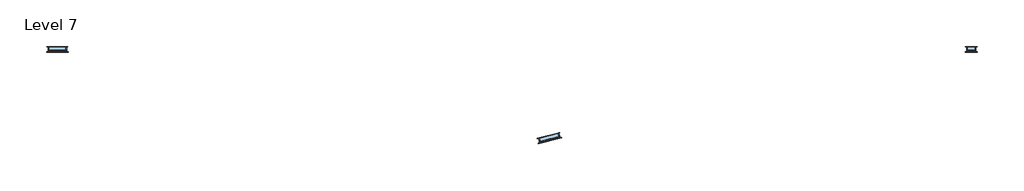
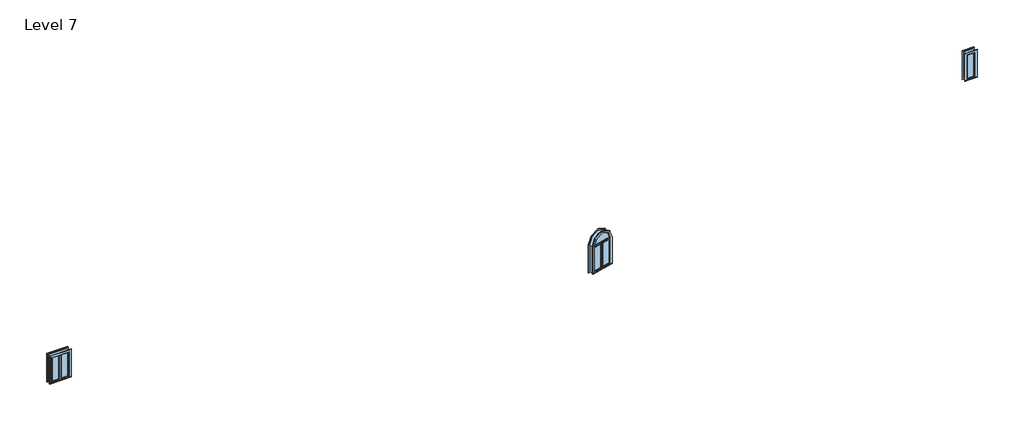
# One storey: 3 windows.
"""IFC4 building model written with IfcOpenShell, lengths in millimetres."""

from ifc_helpers import new_model, si_unit, origin, place, context, project, spatial, transform, mapped, element, save
from components import window_cf4adaea, window_a765b88f, window_bb17773d

model = new_model("IFC4")

# Units and contexts
model_context = context("Model", 3, world=origin())
ifc_project = project(units=[si_unit("LENGTHUNIT", "METRE", prefix="MILLI")], contexts=[model_context])

# Site, building, storey
site = spatial("IfcSite", under=ifc_project)
building = spatial("IfcBuilding", under=site)
storey = spatial("IfcBuildingStorey", under=building, Name="Level 7", Elevation=12801.6)

# Windows
placement = place(None, origin())
window_shape = window_cf4adaea(model_context)
element("IfcWindow", 1, ObjectType="36\" x 48\"", at=placement, inside=storey, context=model_context, shape_type="MappedRepresentation", body=[
    mapped(window_shape, transform((2703.5095295, -16265.2290786, 12801.6), x_axis=(-0.9678343520911785, -0.251588288503755, 0.0), y_axis=(0.251588288503755, -0.9678343520911785, 0.0), z_axis=(0.0, 0.0, 1.0))),
])
window_2_shape = window_a765b88f(model_context)
element("IfcWindow", 2, ObjectType="Awning with Trim : 16\" x 48\"", at=placement, inside=storey, context=model_context, shape_type="MappedRepresentation", body=[
    mapped(window_2_shape, transform((21273.414721, -12354.7237084, 12801.6), x_axis=(-1.0, 0.0, 0.0), y_axis=(0.0, -1.0, 0.0), z_axis=(0.0, 0.0, 1.0))),
])
window_3_shape = window_bb17773d(model_context)
element("IfcWindow", 3, ObjectType="Casement Dbl with Trim : 32\" x 48\"", at=placement, inside=storey, context=model_context, shape_type="MappedRepresentation", body=[
    mapped(window_3_shape, transform((-18960.185279, -12335.6737084, 12801.6), x_axis=(-1.0, 0.0, 0.0), y_axis=(0.0, -1.0, 0.0), z_axis=(0.0, 0.0, 1.0))),
])

save(model, "model.ifc")

# Revit data of these elements
# Type "36\" x 48\""
#   Type Mark = "38"
#   Construction Type Id = "SGL"
#   Assembly Code = "B2020100"
#   Analytic Construction = "Large single-glazed windows"
#   Visual Light Transmittance = 0.9
#   Solar Heat Gain Coefficient = 0.86
#   Heat Transfer Coefficient (U) = 0.979472 BTU/(h·ft²·°F)
#   Height = 4' - 0"
#   Default Sill Height = 3' - 0"
#   Trim Projection - Ext. = 0' - 0 1/2"
#   Trim Projection - Int. = 0' - 0 3/4"
#   Trim Width - Exterior = 0' - 3 1/2"
#   Trim Width - Interior = 0' - 3 1/2"
#   Width = 3' - 0"
#   Window Inset = 0' - 0 3/4"
#   Define Thermal Properties by = 1
#   Glass Pane Material = Glass
#   Sash Material = Sash
#   Trim Exterior Material = Trim
#   Trim Interior Material = Trim
#   Wall Closure = (empty or 0)
# Type "Awning with Trim : 16\" x 48\""
#   Type Mark = "14"
#   Construction Type Id = "GSP4R"
#   Assembly Code = "B2020100"
#   Analytic Construction = "1/8 in Pilkington single glazing"
#   Visual Light Transmittance = 0.9
#   Solar Heat Gain Coefficient = 0.78
#   Heat Transfer Coefficient (U) = 0.6496 BTU/(h·ft²·°F)
#   Height = 4' - 0"
#   Default Sill Height = 3' - 0"
#   Trim Projection - Ext. = 0' - 0 1/2"
#   Trim Projection - Int. = 0' - 0 3/4"
#   Trim Width - Exterior = 0' - 3 1/2"
#   Trim Width - Interior = 0' - 3 1/2"
#   Width = 1' - 4"
#   Window Inset = 0' - 0 3/4"
#   Define Thermal Properties by = 1
#   Glass Pane Material = Glass
#   Sash Material = Sash
#   Trim Exterior Material = Trim
#   Trim Interior Material = Trim
#   Wall Closure = (empty or 0)
# Type "Casement Dbl with Trim : 32\" x 48\""
#   Type Mark = "36"
#   Construction Type Id = "GSP4R"
#   Assembly Code = "B2020100"
#   Analytic Construction = "1/8 in Pilkington single glazing"
#   Visual Light Transmittance = 0.9
#   Solar Heat Gain Coefficient = 0.78
#   Heat Transfer Coefficient (U) = 0.6496 BTU/(h·ft²·°F)
#   Height = 4' - 0"
#   Default Sill Height = 3' - 0"
#   Trim Projection - Ext. = 0' - 0 1/2"
#   Trim Projection - Int. = 0' - 0 3/4"
#   Trim Width - Exterior = 0' - 3 1/2"
#   Trim Width - Interior = 0' - 3 1/2"
#   Width = 2' - 8"
#   Window Inset = 0' - 0 3/4"
#   Define Thermal Properties by = 1
#   Glass Pane Material = Glass
#   Sash Material = Sash
#   Trim Exterior Material = Trim
#   Trim Interior Material = Trim
#   Wall Closure = (empty or 0)
# Element 1 (IfcWindow, "36\" x 48\"")
#   Mark = "30"
#   Phase Created = New Construction
#   Materials on its faces: "Sash", "Trim", "Glass"
# Element 2 (IfcWindow, "Awning with Trim : 16\" x 48\"")
#   Mark = "64"
#   Phase Created = New Construction
#   Materials on its faces: "Sash", "Trim", "Glass"
# Element 3 (IfcWindow, "Casement Dbl with Trim : 32\" x 48\"")
#   Mark = "47"
#   Phase Created = New Construction
#   Materials on its faces: "Sash", "Trim", "Glass"
# Materials
#   "Glass": class "Glass", colour RGB 0 128 192, transparency 0.75, Description = "Soda Lime Glass", Cost = 0
#   "Sash": class "Wood", colour RGB 224 178 126, transparency 0
#   "Trim": class "Wood", colour RGB 224 178 126, transparency 0
